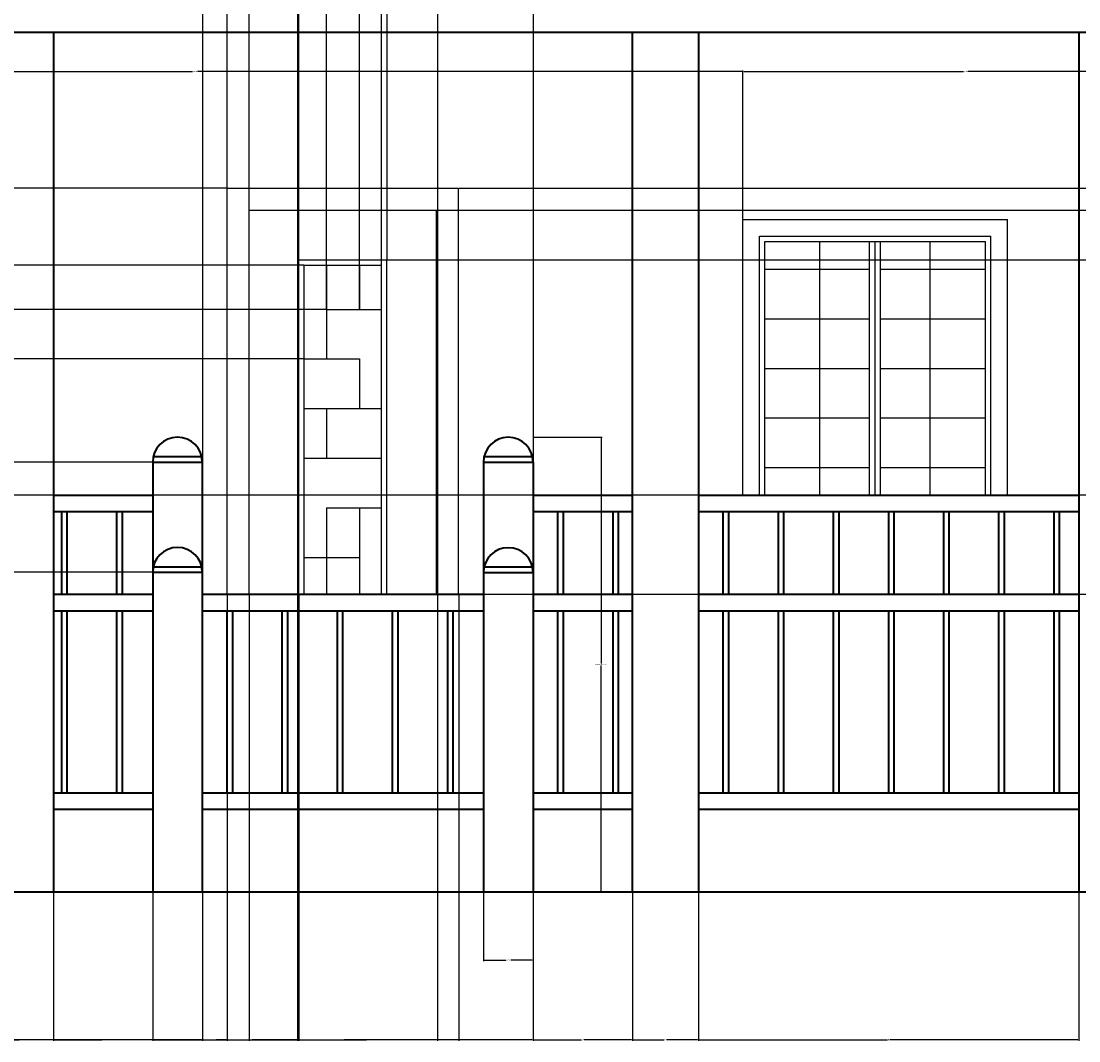
# Model space of a CAD drawing. Units: inches. Extents: x 2154 to 2740, y 571 to 1084.
# Tile 6 of 13: x 2384 to 2576, y 571 to 756. Entities that reach past the tile are written whole.
import ezdxf

# ---------------------------------------------------------------- set-up
doc = ezdxf.new("R2010")
doc.units = ezdxf.units.IN
for name, color, linetype, lineweight in [('A-ANNO-DIMS', 2, 'Continuous', 18), ('A-DOOR', 3, 'Continuous', 25), ('A-ELEV', 7, 'Continuous', 35), ('A-GLAZ', 4, 'Continuous', 25)]:
    doc.layers.add(name, color=color, linetype=linetype, lineweight=lineweight)
doc.styles.get("Standard").update_dxf_attribs({"font": 'arial.ttf'})
doc.dimstyles.get("Standard").update_dxf_attribs({"dimtxt": 0.18, "dimasz": 0.18, "dimexe": 0.18, "dimexo": 0.0625, "dimgap": 0.09, "dimtad": 0, "dimtih": 1, "dimtoh": 1, "dimdec": 4, "dimzin": 0, "dimdsep": 46, "dimtxsty": 'Standard', "dimcen": 0.09, "dimadec": 0, "dimazin": 0, "dimtfac": 1, "dimtdec": 4, "dimtofl": 0, "dimtmove": 0, "dimatfit": 3, "dimfxl": 1, "dimtolj": 1, "dimtzin": 0, "dimarcsym": 0})

# ---------------------------------------------------------------- blocks, each defined once
blk = doc.blocks.new('WIN-ELEV-1200')
for p, q in [((0, 50), (48, 50)), ((0, 0), (0, 50)), ((48, 0), (48, 50)), ((3, 0), (3, 47)), ((3, 47), (45, 47)), ((45, 0), (45, 47)), ((4, 46), (44, 46)), ((4, 0), (4, 46)), ((14, 0), (14, 46)), ((23, 0), (23, 46)), ((24, 0), (24, 46)), ((25, 0), (25, 46)), ((34, 0), (34, 46)), ((44, 0), (44, 46)), ((4, 41), (23, 41)), ((25, 41), (44, 41)), ((4, 32), (23, 32)), ((25, 32), (44, 32)), ((4, 23), (23, 23)), ((25, 23), (44, 23)), ((4, 14), (23, 14)), ((25, 14), (44, 14)), ((4, 5), (23, 5)), ((25, 5), (44, 5))]:
    blk.add_line(p, q)
blk = doc.blocks.new('GATE-POST')
for p, q in [((0, 78), (0, 0)), ((0, 78), (9, 78)), ((9, 78), (9, 0))]:
    blk.add_line(p, q)
blk.add_arc((4.5, 78), 4.5, 0, 180)
blk = doc.blocks.new('*D5')
at = {"layer": 'A-ANNO-DIMS', "color": 0, "lineweight": -2, "transparency": 16777216}
for p, q in [((2477.27, 680.03), (2489.76, 680.03)), ((2489.58, 679.85), (2489.58, 638.97)), ((2489.58, 597.71), (2489.58, 638.6)), ((2477.27, 597.53), (2489.76, 597.53))]:
    blk.add_line(p, q, dxfattribs=at)
at = {"layer": 'A-ANNO-DIMS', "color": 0, "transparency": 16777216}
for points in [[(2489.55, 679.85), (2489.61, 679.85), (2489.58, 680.03)], [(2489.55, 597.71), (2489.61, 597.71), (2489.58, 597.53)]]:
    blk.add_solid(points, dxfattribs=at)
at = {"layer": 'Defpoints', "color": 0, "transparency": 16777216}
for p in [(2477.21, 680.03), (2489.58, 680.03), (2477.21, 597.53)]:
    blk.add_point(p, dxfattribs=at)
at = {"layer": 'A-ANNO-DIMS', "color": 0, "transparency": 16777216, "insert": (2489.58, 638.78), "char_height": 0.18, "attachment_point": 5}
blk.add_mtext('\\A1;GATE POST 83 TYP.', dxfattribs=at)
blk = doc.blocks.new('*D6')
at = {"layer": 'A-ANNO-DIMS', "color": 0, "lineweight": -2, "transparency": 16777216}
for p, q in [((2468.21, 597.47), (2468.21, 584.98)), ((2477.21, 597.47), (2477.21, 584.98)), ((2468.39, 585.16), (2472.25, 585.16)), ((2477.03, 585.16), (2473.16, 585.16))]:
    blk.add_line(p, q, dxfattribs=at)
at = {"layer": 'A-ANNO-DIMS', "color": 0, "transparency": 16777216}
for points in [[(2468.39, 585.19), (2468.39, 585.13), (2468.21, 585.16)], [(2477.03, 585.19), (2477.03, 585.13), (2477.21, 585.16)]]:
    blk.add_solid(points, dxfattribs=at)
at = {"layer": 'Defpoints', "color": 0, "transparency": 16777216}
for p in [(2468.21, 597.53), (2477.21, 597.53), (2477.21, 585.16)]:
    blk.add_point(p, dxfattribs=at)
at = {"layer": 'A-ANNO-DIMS', "color": 0, "transparency": 16777216, "insert": (2472.71, 585.16), "char_height": 0.18, "attachment_point": 5}
blk.add_mtext('\\A1;9 TYP.', dxfattribs=at)
blk = doc.blocks.new('*D9')
at = {"layer": 'A-ANNO-DIMS', "color": 0, "lineweight": -2, "transparency": 16777216}
for p, q in [((2417.21, 970.47), (2417.21, 570.5)), ((2477.21, 970.47), (2477.21, 570.5)), ((2417.39, 570.68), (2446.99, 570.68)), ((2477.03, 570.68), (2447.43, 570.68))]:
    blk.add_line(p, q, dxfattribs=at)
at = {"layer": 'A-ANNO-DIMS', "color": 0, "transparency": 16777216}
for points in [[(2417.39, 570.71), (2417.39, 570.65), (2417.21, 570.68)], [(2477.03, 570.71), (2477.03, 570.65), (2477.21, 570.68)]]:
    blk.add_solid(points, dxfattribs=at)
at = {"layer": 'Defpoints', "color": 0, "transparency": 16777216}
for p in [(2417.21, 970.53), (2477.21, 970.53), (2477.21, 570.68)]:
    blk.add_point(p, dxfattribs=at)
at = {"layer": 'A-ANNO-DIMS', "color": 0, "transparency": 16777216, "insert": (2447.21, 570.68), "char_height": 0.18, "attachment_point": 5}
blk.add_mtext('\\A1;60', dxfattribs=at)
blk = doc.blocks.new('*D10')
at = {"layer": 'A-ANNO-DIMS', "color": 0, "lineweight": -2, "transparency": 16777216}
for p, q in [((2447.14, 1057.01), (2154.18, 1057.01)), ((2154.36, 1056.83), (2154.36, 827.45)), ((2154.36, 597.71), (2154.36, 827.09)), ((2181.14, 597.53), (2154.18, 597.53))]:
    blk.add_line(p, q, dxfattribs=at)
at = {"layer": 'A-ANNO-DIMS', "color": 0, "transparency": 16777216}
for points in [[(2154.33, 1056.83), (2154.39, 1056.83), (2154.36, 1057.01)], [(2154.33, 597.71), (2154.39, 597.71), (2154.36, 597.53)]]:
    blk.add_solid(points, dxfattribs=at)
at = {"layer": 'Defpoints', "color": 0, "transparency": 16777216}
for p in [(2154.36, 1057.01), (2447.21, 1057.01), (2181.21, 597.53)]:
    blk.add_point(p, dxfattribs=at)
at = {"layer": 'A-ANNO-DIMS', "color": 0, "transparency": 16777216, "insert": (2154.36, 827.27), "char_height": 0.18, "attachment_point": 5}
blk.add_mtext('\\A1;459.5', dxfattribs=at)
blk = doc.blocks.new('*D20')
at = {"layer": 'A-ANNO-DIMS', "color": 0, "lineweight": -2, "transparency": 16777216}
for p, q in [((2378.21, 597.47), (2378.21, 570.5)), ((2390.21, 597.47), (2390.21, 570.5)), ((2378.39, 570.68), (2384, 570.68)), ((2390.03, 570.68), (2384.42, 570.68))]:
    blk.add_line(p, q, dxfattribs=at)
at = {"layer": 'A-ANNO-DIMS', "color": 0, "transparency": 16777216}
for points in [[(2378.39, 570.71), (2378.39, 570.65), (2378.21, 570.68)], [(2390.03, 570.71), (2390.03, 570.65), (2390.21, 570.68)]]:
    blk.add_solid(points, dxfattribs=at)
at = {"layer": 'Defpoints', "color": 0, "transparency": 16777216}
for p in [(2378.21, 597.53), (2390.21, 597.53), (2390.21, 570.68)]:
    blk.add_point(p, dxfattribs=at)
at = {"layer": 'A-ANNO-DIMS', "color": 0, "transparency": 16777216, "insert": (2384.21, 570.68), "char_height": 0.18, "attachment_point": 5}
blk.add_mtext('\\A1;12', dxfattribs=at)
blk = doc.blocks.new('*D21')
at = {"layer": 'A-ANNO-DIMS', "color": 0, "lineweight": -2, "transparency": 16777216}
for p, q in [((2390.21, 597.47), (2390.21, 570.5)), ((2408.21, 597.47), (2408.21, 570.5)), ((2390.39, 570.68), (2399, 570.68)), ((2408.03, 570.68), (2399.42, 570.68))]:
    blk.add_line(p, q, dxfattribs=at)
at = {"layer": 'A-ANNO-DIMS', "color": 0, "transparency": 16777216}
for points in [[(2390.39, 570.71), (2390.39, 570.65), (2390.21, 570.68)], [(2408.03, 570.71), (2408.03, 570.65), (2408.21, 570.68)]]:
    blk.add_solid(points, dxfattribs=at)
at = {"layer": 'Defpoints', "color": 0, "transparency": 16777216}
for p in [(2390.21, 597.53), (2408.21, 597.53), (2408.21, 570.68)]:
    blk.add_point(p, dxfattribs=at)
at = {"layer": 'A-ANNO-DIMS', "color": 0, "transparency": 16777216, "insert": (2399.21, 570.68), "char_height": 0.18, "attachment_point": 5}
blk.add_mtext('\\A1;18', dxfattribs=at)
blk = doc.blocks.new('*D22')
at = {"layer": 'A-ANNO-DIMS', "color": 0, "lineweight": -2, "transparency": 16777216}
for p, q in [((2408.21, 597.47), (2408.21, 570.5)), ((2477.21, 597.47), (2477.21, 570.5)), ((2408.39, 570.68), (2442.49, 570.68)), ((2477.03, 570.68), (2442.93, 570.68))]:
    blk.add_line(p, q, dxfattribs=at)
at = {"layer": 'A-ANNO-DIMS', "color": 0, "transparency": 16777216}
for points in [[(2408.39, 570.71), (2408.39, 570.65), (2408.21, 570.68)], [(2477.03, 570.71), (2477.03, 570.65), (2477.21, 570.68)]]:
    blk.add_solid(points, dxfattribs=at)
at = {"layer": 'Defpoints', "color": 0, "transparency": 16777216}
for p in [(2408.21, 597.53), (2477.21, 597.53), (2477.21, 570.68)]:
    blk.add_point(p, dxfattribs=at)
at = {"layer": 'A-ANNO-DIMS', "color": 0, "transparency": 16777216, "insert": (2442.71, 570.68), "char_height": 0.18, "attachment_point": 5}
blk.add_mtext('\\A1;69', dxfattribs=at)
blk = doc.blocks.new('*D23')
at = {"layer": 'A-ANNO-DIMS', "color": 0, "lineweight": -2, "transparency": 16777216}
for p, q in [((2477.21, 597.47), (2477.21, 570.5)), ((2495.21, 597.47), (2495.21, 570.5)), ((2477.39, 570.68), (2486, 570.68)), ((2495.03, 570.68), (2486.42, 570.68))]:
    blk.add_line(p, q, dxfattribs=at)
at = {"layer": 'A-ANNO-DIMS', "color": 0, "transparency": 16777216}
for points in [[(2477.39, 570.71), (2477.39, 570.65), (2477.21, 570.68)], [(2495.03, 570.71), (2495.03, 570.65), (2495.21, 570.68)]]:
    blk.add_solid(points, dxfattribs=at)
at = {"layer": 'Defpoints', "color": 0, "transparency": 16777216}
for p in [(2477.21, 597.53), (2495.21, 597.53), (2495.21, 570.68)]:
    blk.add_point(p, dxfattribs=at)
at = {"layer": 'A-ANNO-DIMS', "color": 0, "transparency": 16777216, "insert": (2486.21, 570.68), "char_height": 0.18, "attachment_point": 5}
blk.add_mtext('\\A1;18', dxfattribs=at)
blk = doc.blocks.new('*D24')
at = {"layer": 'A-ANNO-DIMS', "color": 0, "lineweight": -2, "transparency": 16777216}
for p, q in [((2495.21, 597.47), (2495.21, 570.5)), ((2507.21, 597.47), (2507.21, 570.5)), ((2495.39, 570.68), (2501, 570.68)), ((2507.03, 570.68), (2501.42, 570.68))]:
    blk.add_line(p, q, dxfattribs=at)
at = {"layer": 'A-ANNO-DIMS', "color": 0, "transparency": 16777216}
for points in [[(2495.39, 570.71), (2495.39, 570.65), (2495.21, 570.68)], [(2507.03, 570.71), (2507.03, 570.65), (2507.21, 570.68)]]:
    blk.add_solid(points, dxfattribs=at)
at = {"layer": 'Defpoints', "color": 0, "transparency": 16777216}
for p in [(2495.21, 597.53), (2507.21, 597.53), (2507.21, 570.68)]:
    blk.add_point(p, dxfattribs=at)
at = {"layer": 'A-ANNO-DIMS', "color": 0, "transparency": 16777216, "insert": (2501.21, 570.68), "char_height": 0.18, "attachment_point": 5}
blk.add_mtext('\\A1;12', dxfattribs=at)
blk = doc.blocks.new('*D25')
at = {"layer": 'A-ANNO-DIMS', "color": 0, "lineweight": -2, "transparency": 16777216}
for p, q in [((2507.21, 597.47), (2507.21, 570.5)), ((2576.21, 597.47), (2576.21, 570.5)), ((2507.39, 570.68), (2541.49, 570.68)), ((2576.03, 570.68), (2541.93, 570.68))]:
    blk.add_line(p, q, dxfattribs=at)
at = {"layer": 'A-ANNO-DIMS', "color": 0, "transparency": 16777216}
for points in [[(2507.39, 570.71), (2507.39, 570.65), (2507.21, 570.68)], [(2576.03, 570.71), (2576.03, 570.65), (2576.21, 570.68)]]:
    blk.add_solid(points, dxfattribs=at)
at = {"layer": 'Defpoints', "color": 0, "transparency": 16777216}
for p in [(2507.21, 597.53), (2576.21, 597.53), (2576.21, 570.68)]:
    blk.add_point(p, dxfattribs=at)
at = {"layer": 'A-ANNO-DIMS', "color": 0, "transparency": 16777216, "insert": (2541.71, 570.68), "char_height": 0.18, "attachment_point": 5}
blk.add_mtext('\\A1;69', dxfattribs=at)
blk = doc.blocks.new('*D29')
at = {"layer": 'A-ANNO-DIMS', "color": 0, "lineweight": -2, "transparency": 16777216}
for p, q in [((2657.14, 669.53), (2154.18, 669.53)), ((2154.36, 669.35), (2154.36, 633.71)), ((2154.36, 597.71), (2154.36, 633.35)), ((2657.14, 597.53), (2154.18, 597.53))]:
    blk.add_line(p, q, dxfattribs=at)
at = {"layer": 'A-ANNO-DIMS', "color": 0, "transparency": 16777216}
for points in [[(2154.33, 669.35), (2154.39, 669.35), (2154.36, 669.53)], [(2154.33, 597.71), (2154.39, 597.71), (2154.36, 597.53)]]:
    blk.add_solid(points, dxfattribs=at)
at = {"layer": 'Defpoints', "color": 0, "transparency": 16777216}
for p in [(2154.36, 669.53), (2657.21, 669.53), (2657.21, 597.53)]:
    blk.add_point(p, dxfattribs=at)
at = {"layer": 'A-ANNO-DIMS', "color": 0, "transparency": 16777216, "insert": (2154.36, 633.53), "char_height": 0.18, "attachment_point": 5}
blk.add_mtext('\\A1;72', dxfattribs=at)
blk = doc.blocks.new('*D31')
at = {"layer": 'A-ANNO-DIMS', "color": 0, "lineweight": -2, "transparency": 16777216}
for p, q in [((2421.64, 725.23), (2154.18, 725.23)), ((2154.36, 725.05), (2154.36, 661.56)), ((2154.36, 597.71), (2154.36, 661.2)), ((2417.14, 597.53), (2154.18, 597.53))]:
    blk.add_line(p, q, dxfattribs=at)
at = {"layer": 'A-ANNO-DIMS', "color": 0, "transparency": 16777216}
for points in [[(2154.33, 725.05), (2154.39, 725.05), (2154.36, 725.23)], [(2154.33, 597.71), (2154.39, 597.71), (2154.36, 597.53)]]:
    blk.add_solid(points, dxfattribs=at)
at = {"layer": 'Defpoints', "color": 0, "transparency": 16777216}
for p in [(2154.36, 725.23), (2421.71, 725.23), (2417.21, 597.53)]:
    blk.add_point(p, dxfattribs=at)
at = {"layer": 'A-ANNO-DIMS', "color": 0, "transparency": 16777216, "insert": (2154.36, 661.38), "char_height": 0.18, "attachment_point": 5}
blk.add_mtext('\\A1;127.7', dxfattribs=at)
blk = doc.blocks.new('*D39')
at = {"layer": 'A-ANNO-DIMS', "color": 0, "lineweight": -2, "transparency": 16777216}
for p, q in [((2183.21, 979.47), (2183.21, 570.5)), ((2417.21, 970.47), (2417.21, 570.5)), ((2183.39, 570.68), (2299.92, 570.68)), ((2417.03, 570.68), (2300.5, 570.68))]:
    blk.add_line(p, q, dxfattribs=at)
at = {"layer": 'A-ANNO-DIMS', "color": 0, "transparency": 16777216}
for points in [[(2183.39, 570.71), (2183.39, 570.65), (2183.21, 570.68)], [(2417.03, 570.71), (2417.03, 570.65), (2417.21, 570.68)]]:
    blk.add_solid(points, dxfattribs=at)
at = {"layer": 'Defpoints', "color": 0, "transparency": 16777216}
for p in [(2183.21, 979.53), (2417.21, 970.53), (2417.21, 570.68)]:
    blk.add_point(p, dxfattribs=at)
at = {"layer": 'A-ANNO-DIMS', "color": 0, "transparency": 16777216, "insert": (2300.21, 570.68), "char_height": 0.18, "attachment_point": 5}
blk.add_mtext('\\A1;234', dxfattribs=at)
blk = doc.blocks.new('*D44')
at = {"layer": 'A-ANNO-DIMS', "color": 0, "lineweight": -2, "transparency": 16777216}
for p, q in [((2316.5, 719.59), (2316.5, 746.56)), ((2316.68, 746.38), (2415.42, 746.38)), ((2515.07, 746.38), (2416.33, 746.38)), ((2515.25, 719.59), (2515.25, 746.56))]:
    blk.add_line(p, q, dxfattribs=at)
at = {"layer": 'A-ANNO-DIMS', "color": 0, "transparency": 16777216}
for points in [[(2316.68, 746.41), (2316.68, 746.35), (2316.5, 746.38)], [(2515.07, 746.41), (2515.07, 746.35), (2515.25, 746.38)]]:
    blk.add_solid(points, dxfattribs=at)
at = {"layer": 'Defpoints', "color": 0, "transparency": 16777216}
for p in [(2515.25, 746.38), (2316.5, 719.53), (2515.25, 719.53)]:
    blk.add_point(p, dxfattribs=at)
at = {"layer": 'A-ANNO-DIMS', "color": 0, "transparency": 16777216, "insert": (2415.87, 746.38), "char_height": 0.18, "attachment_point": 5}
blk.add_mtext('\\A1;198.75', dxfattribs=at)
blk = doc.blocks.new('*D45')
at = {"layer": 'A-ANNO-DIMS', "color": 0, "lineweight": -2, "transparency": 16777216}
for p, q in [((2515.25, 719.59), (2515.25, 746.56)), ((2515.43, 746.38), (2555.29, 746.38)), ((2595.93, 746.38), (2556.07, 746.38)), ((2596.11, 719.59), (2596.11, 746.56))]:
    blk.add_line(p, q, dxfattribs=at)
at = {"layer": 'A-ANNO-DIMS', "color": 0, "transparency": 16777216}
for points in [[(2515.43, 746.41), (2515.43, 746.35), (2515.25, 746.38)], [(2595.93, 746.41), (2595.93, 746.35), (2596.11, 746.38)]]:
    blk.add_solid(points, dxfattribs=at)
at = {"layer": 'Defpoints', "color": 0, "transparency": 16777216}
for p in [(2596.11, 746.38), (2515.25, 719.53), (2596.11, 719.53)]:
    blk.add_point(p, dxfattribs=at)
at = {"layer": 'A-ANNO-DIMS', "color": 0, "transparency": 16777216, "insert": (2555.68, 746.38), "char_height": 0.18, "attachment_point": 5}
blk.add_mtext('\\A1;80.86', dxfattribs=at)
blk = doc.blocks.new('*D75')
at = {"layer": 'A-ANNO-DIMS', "color": 0, "lineweight": -2, "transparency": 16777216}
for p, q in [((2434.46, 990.57), (2434.46, 570.5)), ((2417.21, 981.47), (2417.21, 570.5)), ((2417.39, 570.68), (2425.45, 570.68)), ((2434.28, 570.68), (2426.22, 570.68))]:
    blk.add_line(p, q, dxfattribs=at)
at = {"layer": 'A-ANNO-DIMS', "color": 0, "transparency": 16777216}
for points in [[(2417.39, 570.71), (2417.39, 570.65), (2417.21, 570.68)], [(2434.28, 570.71), (2434.28, 570.65), (2434.46, 570.68)]]:
    blk.add_solid(points, dxfattribs=at)
at = {"layer": 'Defpoints', "color": 0, "transparency": 16777216}
for p in [(2434.46, 990.64), (2417.21, 981.53), (2434.46, 570.68)]:
    blk.add_point(p, dxfattribs=at)
at = {"layer": 'A-ANNO-DIMS', "color": 0, "transparency": 16777216, "insert": (2425.83, 570.68), "char_height": 0.18, "attachment_point": 5}
blk.add_mtext('\\A1;17.25', dxfattribs=at)
blk = doc.blocks.new('*D76')
at = {"layer": 'A-ANNO-DIMS', "color": 0, "lineweight": -2, "transparency": 16777216}
for p, q in [((2434.46, 990.57), (2434.46, 570.5)), ((2459.89, 990.57), (2459.89, 570.5)), ((2434.64, 570.68), (2446.71, 570.68)), ((2459.71, 570.68), (2447.64, 570.68))]:
    blk.add_line(p, q, dxfattribs=at)
at = {"layer": 'A-ANNO-DIMS', "color": 0, "transparency": 16777216}
for points in [[(2434.64, 570.71), (2434.64, 570.65), (2434.46, 570.68)], [(2459.71, 570.71), (2459.71, 570.65), (2459.89, 570.68)]]:
    blk.add_solid(points, dxfattribs=at)
at = {"layer": 'Defpoints', "color": 0, "transparency": 16777216}
for p in [(2434.46, 990.64), (2459.89, 990.64), (2459.89, 570.68)]:
    blk.add_point(p, dxfattribs=at)
at = {"layer": 'A-ANNO-DIMS', "color": 0, "transparency": 16777216, "insert": (2447.17, 570.68), "char_height": 0.18, "attachment_point": 5}
blk.add_mtext('\\A1;25.433', dxfattribs=at)
blk = doc.blocks.new('*D86')
at = {"layer": 'A-ANNO-DIMS', "color": 0, "lineweight": -2, "transparency": 16777216}
for p, q in [((2421.71, 651.47), (2421.71, 570.5)), ((2463.71, 651.47), (2463.71, 570.5)), ((2421.89, 570.68), (2442.49, 570.68)), ((2463.53, 570.68), (2442.93, 570.68))]:
    blk.add_line(p, q, dxfattribs=at)
at = {"layer": 'A-ANNO-DIMS', "color": 0, "transparency": 16777216}
for points in [[(2421.89, 570.71), (2421.89, 570.65), (2421.71, 570.68)], [(2463.53, 570.71), (2463.53, 570.65), (2463.71, 570.68)]]:
    blk.add_solid(points, dxfattribs=at)
at = {"layer": 'Defpoints', "color": 0, "transparency": 16777216}
for p in [(2421.71, 651.53), (2463.71, 651.53), (2463.71, 570.68)]:
    blk.add_point(p, dxfattribs=at)
at = {"layer": 'A-ANNO-DIMS', "color": 0, "transparency": 16777216, "insert": (2442.71, 570.68), "char_height": 0.18, "attachment_point": 5}
blk.add_mtext('\\A1;42', dxfattribs=at)
blk = doc.blocks.new('*D87')
at = {"layer": 'A-ANNO-DIMS', "color": 0, "lineweight": -2, "transparency": 16777216}
for p, q in [((2421.71, 725.29), (2421.71, 1084.04)), ((2425.71, 721.29), (2425.71, 1084.04)), ((2421.89, 1083.86), (2423.55, 1083.86)), ((2425.53, 1083.86), (2423.86, 1083.86))]:
    blk.add_line(p, q, dxfattribs=at)
at = {"layer": 'A-ANNO-DIMS', "color": 0, "transparency": 16777216}
for points in [[(2421.89, 1083.89), (2421.89, 1083.83), (2421.71, 1083.86)], [(2425.53, 1083.89), (2425.53, 1083.83), (2425.71, 1083.86)]]:
    blk.add_solid(points, dxfattribs=at)
at = {"layer": 'Defpoints', "color": 0, "transparency": 16777216}
for p in [(2425.71, 1083.86), (2421.71, 725.23), (2425.71, 721.23)]:
    blk.add_point(p, dxfattribs=at)
at = {"layer": 'A-ANNO-DIMS', "color": 0, "transparency": 16777216, "insert": (2423.71, 1083.86), "char_height": 0.18, "attachment_point": 5}
blk.add_mtext('\\A1;4', dxfattribs=at)
blk = doc.blocks.new('*D88')
at = {"layer": 'A-ANNO-DIMS', "color": 0, "lineweight": -2, "transparency": 16777216}
for p, q in [((2463.769199, 725.228066), (2740.236699, 725.228066)), ((2740.056699, 725.048066), (2740.056699, 723.408066)), ((2740.056699, 721.408066), (2740.056699, 723.048066)), ((2459.769199, 721.228066), (2740.236699, 721.228066))]:
    blk.add_line(p, q, dxfattribs=at)
at = {"layer": 'A-ANNO-DIMS', "color": 0, "transparency": 16777216}
for points in [[(2740.026699, 725.048066), (2740.086699, 725.048066), (2740.056699, 725.228066)], [(2740.026699, 721.408066), (2740.086699, 721.408066), (2740.056699, 721.228066)]]:
    blk.add_solid(points, dxfattribs=at)
at = {"layer": 'Defpoints', "color": 0, "transparency": 16777216}
for p in [(2463.706699, 725.228066), (2740.056699, 725.228066), (2459.706699, 721.228066)]:
    blk.add_point(p, dxfattribs=at)
at = {"layer": 'A-ANNO-DIMS', "color": 0, "transparency": 16777216, "insert": (2740.056699, 723.228066), "char_height": 0.18, "attachment_point": 5}
blk.add_mtext('\\A1;4', dxfattribs=at)
blk = doc.blocks.new('*D89')
at = {"layer": 'A-ANNO-DIMS', "color": 0, "lineweight": -2, "transparency": 16777216}
for p, q in [((2425.71, 651.47), (2425.71, 570.5)), ((2434.71, 651.47), (2434.71, 570.5)), ((2425.89, 570.68), (2430.06, 570.68)), ((2434.53, 570.68), (2430.36, 570.68))]:
    blk.add_line(p, q, dxfattribs=at)
at = {"layer": 'A-ANNO-DIMS', "color": 0, "transparency": 16777216}
for points in [[(2425.89, 570.71), (2425.89, 570.65), (2425.71, 570.68)], [(2434.53, 570.71), (2434.53, 570.65), (2434.71, 570.68)]]:
    blk.add_solid(points, dxfattribs=at)
at = {"layer": 'Defpoints', "color": 0, "transparency": 16777216}
for p in [(2425.71, 651.53), (2434.71, 651.53), (2434.71, 570.68)]:
    blk.add_point(p, dxfattribs=at)
at = {"layer": 'A-ANNO-DIMS', "color": 0, "transparency": 16777216, "insert": (2430.21, 570.68), "char_height": 0.18, "attachment_point": 5}
blk.add_mtext('\\A1;9', dxfattribs=at)
blk = doc.blocks.new('*D90')
at = {"layer": 'A-ANNO-DIMS', "color": 0, "lineweight": -2, "transparency": 16777216}
for p, q in [((2434.71, 712.29), (2434.71, 1084.04)), ((2450.71, 712.29), (2450.71, 1084.04)), ((2434.89, 1083.86), (2442.5, 1083.86)), ((2450.53, 1083.86), (2442.92, 1083.86))]:
    blk.add_line(p, q, dxfattribs=at)
at = {"layer": 'A-ANNO-DIMS', "color": 0, "transparency": 16777216}
for points in [[(2434.89, 1083.89), (2434.89, 1083.83), (2434.71, 1083.86)], [(2450.53, 1083.89), (2450.53, 1083.83), (2450.71, 1083.86)]]:
    blk.add_solid(points, dxfattribs=at)
at = {"layer": 'Defpoints', "color": 0, "transparency": 16777216}
for p in [(2450.71, 1083.86), (2434.71, 712.23), (2450.71, 712.23)]:
    blk.add_point(p, dxfattribs=at)
at = {"layer": 'A-ANNO-DIMS', "color": 0, "transparency": 16777216, "insert": (2442.71, 1083.86), "char_height": 0.18, "attachment_point": 5}
blk.add_mtext('\\A1;16', dxfattribs=at)
blk = doc.blocks.new('*D91')
at = {"layer": 'A-ANNO-DIMS', "color": 0, "lineweight": -2, "transparency": 16777216}
for p, q in [((2450.77, 712.23), (2740.24, 712.23)), ((2740.06, 712.05), (2740.06, 682.06)), ((2740.06, 651.71), (2740.06, 681.7)), ((2450.77, 651.53), (2740.24, 651.53))]:
    blk.add_line(p, q, dxfattribs=at)
at = {"layer": 'A-ANNO-DIMS', "color": 0, "transparency": 16777216}
for points in [[(2740.03, 712.05), (2740.09, 712.05), (2740.06, 712.23)], [(2740.03, 651.71), (2740.09, 651.71), (2740.06, 651.53)]]:
    blk.add_solid(points, dxfattribs=at)
at = {"layer": 'Defpoints', "color": 0, "transparency": 16777216}
for p in [(2450.71, 712.23), (2740.06, 712.23), (2450.71, 651.53)]:
    blk.add_point(p, dxfattribs=at)
at = {"layer": 'A-ANNO-DIMS', "color": 0, "transparency": 16777216, "insert": (2740.06, 681.88), "char_height": 0.18, "attachment_point": 5}
blk.add_mtext('\\A1;60.7', dxfattribs=at)
blk = doc.blocks.new('*D92')
at = {"layer": 'A-ANNO-DIMS', "color": 0, "lineweight": -2, "transparency": 16777216}
for p, q in [((2463.77, 725.23), (2740.24, 725.23)), ((2740.06, 725.05), (2740.06, 688.56)), ((2740.06, 651.71), (2740.06, 688.2)), ((2463.77, 651.53), (2740.24, 651.53))]:
    blk.add_line(p, q, dxfattribs=at)
at = {"layer": 'A-ANNO-DIMS', "color": 0, "transparency": 16777216}
for points in [[(2740.03, 725.05), (2740.09, 725.05), (2740.06, 725.23)], [(2740.03, 651.71), (2740.09, 651.71), (2740.06, 651.53)]]:
    blk.add_solid(points, dxfattribs=at)
at = {"layer": 'Defpoints', "color": 0, "transparency": 16777216}
for p in [(2463.71, 725.23), (2740.06, 725.23), (2463.71, 651.53)]:
    blk.add_point(p, dxfattribs=at)
at = {"layer": 'A-ANNO-DIMS', "color": 0, "transparency": 16777216, "insert": (2740.06, 688.38), "char_height": 0.18, "attachment_point": 5}
blk.add_mtext('\\A1;73.7', dxfattribs=at)
blk = doc.blocks.new('*D93')
at = {"layer": 'A-ANNO-DIMS', "color": 0, "lineweight": -2, "transparency": 16777216}
for p, q in [((2439.71, 703.29), (2439.71, 1084.04)), ((2445.71, 703.29), (2445.71, 1084.04)), ((2439.89, 1083.86), (2442.56, 1083.86)), ((2445.53, 1083.86), (2442.86, 1083.86))]:
    blk.add_line(p, q, dxfattribs=at)
at = {"layer": 'A-ANNO-DIMS', "color": 0, "transparency": 16777216}
for points in [[(2439.89, 1083.89), (2439.89, 1083.83), (2439.71, 1083.86)], [(2445.53, 1083.89), (2445.53, 1083.83), (2445.71, 1083.86)]]:
    blk.add_solid(points, dxfattribs=at)
at = {"layer": 'Defpoints', "color": 0, "transparency": 16777216}
for p in [(2445.71, 1083.86), (2439.71, 703.23), (2445.71, 703.23)]:
    blk.add_point(p, dxfattribs=at)
at = {"layer": 'A-ANNO-DIMS', "color": 0, "transparency": 16777216, "insert": (2442.71, 1083.86), "char_height": 0.18, "attachment_point": 5}
blk.add_mtext('\\A1;6', dxfattribs=at)
blk = doc.blocks.new('*D94')
at = {"layer": 'A-ANNO-DIMS', "color": 0, "lineweight": -2, "transparency": 16777216}
for p, q in [((2445.71, 703.29), (2445.71, 1084.04)), ((2449.71, 703.29), (2449.71, 1084.04)), ((2445.89, 1083.86), (2447.55, 1083.86)), ((2449.53, 1083.86), (2447.86, 1083.86))]:
    blk.add_line(p, q, dxfattribs=at)
at = {"layer": 'A-ANNO-DIMS', "color": 0, "transparency": 16777216}
for points in [[(2445.89, 1083.89), (2445.89, 1083.83), (2445.71, 1083.86)], [(2449.53, 1083.89), (2449.53, 1083.83), (2449.71, 1083.86)]]:
    blk.add_solid(points, dxfattribs=at)
at = {"layer": 'Defpoints', "color": 0, "transparency": 16777216}
for p in [(2449.71, 1083.86), (2445.71, 703.23), (2449.71, 703.23)]:
    blk.add_point(p, dxfattribs=at)
at = {"layer": 'A-ANNO-DIMS', "color": 0, "transparency": 16777216, "insert": (2447.71, 1083.86), "char_height": 0.18, "attachment_point": 5}
blk.add_mtext('\\A1;4', dxfattribs=at)
blk = doc.blocks.new('*D95')
at = {"layer": 'A-ANNO-DIMS', "color": 0, "lineweight": -2, "transparency": 16777216}
for p, q in [((2435.64, 711.23), (2154.18, 711.23)), ((2154.36, 711.05), (2154.36, 707.41)), ((2154.36, 703.41), (2154.36, 707.05)), ((2439.64, 703.23), (2154.18, 703.23))]:
    blk.add_line(p, q, dxfattribs=at)
at = {"layer": 'A-ANNO-DIMS', "color": 0, "transparency": 16777216}
for points in [[(2154.33, 711.05), (2154.39, 711.05), (2154.36, 711.23)], [(2154.33, 703.41), (2154.39, 703.41), (2154.36, 703.23)]]:
    blk.add_solid(points, dxfattribs=at)
at = {"layer": 'Defpoints', "color": 0, "transparency": 16777216}
for p in [(2435.71, 711.23), (2154.36, 703.23), (2439.71, 703.23)]:
    blk.add_point(p, dxfattribs=at)
at = {"layer": 'A-ANNO-DIMS', "color": 0, "transparency": 16777216, "insert": (2154.36, 707.23), "char_height": 0.18, "attachment_point": 5}
blk.add_mtext('\\A1;8', dxfattribs=at)
blk = doc.blocks.new('*D96')
at = {"layer": 'A-ANNO-DIMS', "color": 0, "lineweight": -2, "transparency": 16777216}
for p, q in [((2439.64, 703.23), (2154.18, 703.23)), ((2154.36, 703.05), (2154.36, 698.91)), ((2154.36, 694.41), (2154.36, 698.55)), ((2435.64, 694.23), (2154.18, 694.23))]:
    blk.add_line(p, q, dxfattribs=at)
at = {"layer": 'A-ANNO-DIMS', "color": 0, "transparency": 16777216}
for points in [[(2154.33, 703.05), (2154.39, 703.05), (2154.36, 703.23)], [(2154.33, 694.41), (2154.39, 694.41), (2154.36, 694.23)]]:
    blk.add_solid(points, dxfattribs=at)
at = {"layer": 'Defpoints', "color": 0, "transparency": 16777216}
for p in [(2439.71, 703.23), (2154.36, 694.23), (2435.71, 694.23)]:
    blk.add_point(p, dxfattribs=at)
at = {"layer": 'A-ANNO-DIMS', "color": 0, "transparency": 16777216, "insert": (2154.36, 698.73), "char_height": 0.18, "attachment_point": 5}
blk.add_mtext('\\A1;9', dxfattribs=at)
blk = doc.blocks.new('*D97')
at = {"layer": 'A-ANNO-DIMS', "color": 0, "lineweight": -2, "transparency": 16777216}
for p, q in [((2417.21, 675.47), (2417.21, 570.5)), ((2421.71, 651.47), (2421.71, 570.5)), ((2417.39, 570.68), (2419.2, 570.68)), ((2421.53, 570.68), (2419.71, 570.68))]:
    blk.add_line(p, q, dxfattribs=at)
at = {"layer": 'A-ANNO-DIMS', "color": 0, "transparency": 16777216}
for points in [[(2417.39, 570.71), (2417.39, 570.65), (2417.21, 570.68)], [(2421.53, 570.71), (2421.53, 570.65), (2421.71, 570.68)]]:
    blk.add_solid(points, dxfattribs=at)
at = {"layer": 'Defpoints', "color": 0, "transparency": 16777216}
for p in [(2417.21, 675.53), (2421.71, 651.53), (2421.71, 570.68)]:
    blk.add_point(p, dxfattribs=at)
at = {"layer": 'A-ANNO-DIMS', "color": 0, "transparency": 16777216, "insert": (2419.46, 570.68), "char_height": 0.18, "attachment_point": 5}
blk.add_mtext('\\A1;4.5', dxfattribs=at)
blk = doc.blocks.new('*D98')
at = {"layer": 'A-ANNO-DIMS', "color": 0, "lineweight": -2, "transparency": 16777216}
for p, q in [((2408.14, 675.53), (2154.18, 675.53)), ((2154.36, 675.35), (2154.36, 665.71)), ((2154.36, 655.71), (2154.36, 665.35)), ((2408.14, 655.53), (2154.18, 655.53))]:
    blk.add_line(p, q, dxfattribs=at)
at = {"layer": 'A-ANNO-DIMS', "color": 0, "transparency": 16777216}
for points in [[(2154.33, 675.35), (2154.39, 675.35), (2154.36, 675.53)], [(2154.33, 655.71), (2154.39, 655.71), (2154.36, 655.53)]]:
    blk.add_solid(points, dxfattribs=at)
at = {"layer": 'Defpoints', "color": 0, "transparency": 16777216}
for p in [(2154.36, 675.53), (2408.21, 675.53), (2408.21, 655.53)]:
    blk.add_point(p, dxfattribs=at)
at = {"layer": 'A-ANNO-DIMS', "color": 0, "transparency": 16777216, "insert": (2154.36, 665.53), "char_height": 0.18, "attachment_point": 5}
blk.add_mtext('\\A1;20', dxfattribs=at)

msp = doc.modelspace()

# ---------------------------------------------------------------- linework, layer by layer
at = {"layer": 'A-DOOR'}
for p, q in [((2421.7067, 651.5321), (2421.7067, 725.2281)), ((2421.7067, 725.2281), (2463.7067, 725.2281)), ((2463.7067, 651.5321), (2463.7067, 725.2281)), ((2425.7067, 721.2281), (2459.7067, 721.2281)), ((2425.7067, 651.5321), (2425.7067, 721.2281)), ((2459.7067, 651.5321), (2459.7067, 721.2281)), ((2434.7067, 651.5321), (2434.7067, 712.2281)), ((2434.7067, 712.2281), (2450.7067, 712.2281)), ((2450.7067, 651.5321), (2450.7067, 712.2281)), ((2435.7067, 711.2281), (2449.7067, 711.2281)), ((2435.7067, 651.5321), (2435.7067, 711.2281)), ((2439.7067, 711.2281), (2439.7067, 694.2281)), ((2445.7067, 711.2281), (2445.7067, 703.2281)), ((2449.7067, 651.5321), (2449.7067, 711.2281)), ((2439.7067, 703.2281), (2449.7067, 703.2281)), ((2435.7067, 694.2281), (2445.7067, 694.2281)), ((2445.7067, 694.2281), (2445.7067, 685.2281)), ((2435.7067, 685.2281), (2449.7067, 685.2281)), ((2439.7067, 685.2281), (2439.7067, 676.2281)), ((2435.7067, 676.2281), (2449.7067, 676.2281)), ((2439.7067, 667.2281), (2449.7067, 667.2281)), ((2439.7067, 667.2281), (2439.7067, 651.5321)), ((2445.7067, 667.2281), (2445.7067, 651.5321)), ((2435.7067, 658.2281), (2445.7067, 658.2281))]:
    msp.add_line(p, q, dxfattribs=at)
at = {"layer": 'A-ELEV'}
for p, q in [((2181.2067, 753.5321), (2713.2067, 753.5321)), ((2390.2067, 753.5321), (2390.2067, 597.5321)), ((2495.2067, 753.5321), (2495.2067, 597.5321)), ((2507.2067, 753.5321), (2507.2067, 597.5321)), ((2576.2067, 753.5321), (2576.2067, 597.5321)), ((2408.2067, 676.5321), (2417.2067, 676.5321)), ((2468.2067, 676.5321), (2477.2067, 676.5321)), ((2390.2067, 669.5321), (2408.2067, 669.5321)), ((2477.2067, 669.5321), (2495.2067, 669.5321)), ((2507.2067, 669.5321), (2576.2067, 669.5321)), ((2390.2067, 666.5321), (2408.2067, 666.5321)), ((2391.6527, 666.5321), (2391.6527, 651.5321)), ((2392.6527, 666.5321), (2392.6527, 651.5321)), ((2401.6527, 666.5321), (2401.6527, 651.5321)), ((2402.6527, 666.5321), (2402.6527, 651.5321)), ((2477.2067, 666.5321), (2495.2067, 666.5321)), ((2481.6527, 666.5321), (2481.6527, 651.5321)), ((2482.6527, 666.5321), (2482.6527, 651.5321)), ((2491.6527, 666.5321), (2491.6527, 651.5321)), ((2492.6527, 666.5321), (2492.6527, 651.5321)), ((2507.2067, 666.5321), (2576.2067, 666.5321)), ((2511.6527, 666.5321), (2511.6527, 651.5321)), ((2512.6527, 666.5321), (2512.6527, 651.5321)), ((2521.6527, 666.5321), (2521.6527, 651.5321)), ((2522.6527, 666.5321), (2522.6527, 651.5321)), ((2531.6527, 666.5321), (2531.6527, 651.5321)), ((2532.6527, 666.5321), (2532.6527, 651.5321)), ((2541.6527, 666.5321), (2541.6527, 651.5321)), ((2542.6527, 666.5321), (2542.6527, 651.5321)), ((2551.6527, 666.5321), (2551.6527, 651.5321)), ((2552.6527, 666.5321), (2552.6527, 651.5321)), ((2561.6527, 666.5321), (2561.6527, 651.5321)), ((2562.6527, 666.5321), (2562.6527, 651.5321)), ((2571.6527, 666.5321), (2571.6527, 651.5321)), ((2572.6527, 666.5321), (2572.6527, 651.5321)), ((2408.2067, 656.5321), (2417.2067, 656.5321)), ((2468.2067, 656.4869), (2477.2067, 656.4869)), ((2408.2067, 655.5321), (2417.2067, 655.5321)), ((2468.2067, 655.4869), (2477.2067, 655.4869)), ((2390.2067, 651.5321), (2408.2067, 651.5321)), ((2417.2067, 651.5321), (2468.2067, 651.5321)), ((2477.2067, 651.5321), (2495.2067, 651.5321)), ((2507.2067, 651.5321), (2576.2067, 651.5321)), ((2390.2067, 648.5321), (2408.2067, 648.5321)), ((2391.6527, 648.5321), (2391.6527, 615.5321)), ((2392.6527, 648.5321), (2392.6527, 615.5321)), ((2401.6527, 648.5321), (2401.6527, 615.5321)), ((2402.6527, 648.5321), (2402.6527, 615.5321)), ((2417.2067, 648.5321), (2468.2067, 648.5321)), ((2421.6527, 648.5321), (2421.6527, 615.5321)), ((2422.6527, 648.5321), (2422.6527, 615.5321)), ((2431.6527, 648.5321), (2431.6527, 615.5321)), ((2432.6527, 648.5321), (2432.6527, 615.5321)), ((2441.6527, 648.5321), (2441.6527, 615.5321)), ((2442.6527, 648.5321), (2442.6527, 615.5321)), ((2451.6527, 648.5321), (2451.6527, 615.5321)), ((2452.6527, 648.5321), (2452.6527, 615.5321)), ((2461.6527, 648.5321), (2461.6527, 615.5321)), ((2462.6527, 648.5321), (2462.6527, 615.5321)), ((2477.2067, 648.5321), (2495.2067, 648.5321)), ((2481.6527, 648.5321), (2481.6527, 615.5321)), ((2482.6527, 648.5321), (2482.6527, 615.5321)), ((2491.6527, 648.5321), (2491.6527, 615.5321)), ((2492.6527, 648.5321), (2492.6527, 615.5321)), ((2507.2067, 648.5321), (2576.2067, 648.5321)), ((2511.6527, 648.5321), (2511.6527, 615.5321)), ((2512.6527, 648.5321), (2512.6527, 615.5321)), ((2521.6527, 648.5321), (2521.6527, 615.5321)), ((2522.6527, 648.5321), (2522.6527, 615.5321)), ((2531.6527, 648.5321), (2531.6527, 615.5321)), ((2532.6527, 648.5321), (2532.6527, 615.5321)), ((2541.6527, 648.5321), (2541.6527, 615.5321)), ((2542.6527, 648.5321), (2542.6527, 615.5321)), ((2551.6527, 648.5321), (2551.6527, 615.5321)), ((2552.6527, 648.5321), (2552.6527, 615.5321)), ((2561.6527, 648.5321), (2561.6527, 615.5321)), ((2562.6527, 648.5321), (2562.6527, 615.5321)), ((2571.6527, 648.5321), (2571.6527, 615.5321)), ((2572.6527, 648.5321), (2572.6527, 615.5321)), ((2390.2067, 615.5321), (2408.2067, 615.5321)), ((2417.2067, 615.5321), (2468.2067, 615.5321)), ((2477.2067, 615.5321), (2495.2067, 615.5321)), ((2507.2067, 615.5321), (2576.2067, 615.5321)), ((2390.2067, 612.5321), (2408.2067, 612.5321)), ((2417.2067, 612.5321), (2468.2067, 612.5321)), ((2477.2067, 612.5321), (2495.2067, 612.5321)), ((2507.2067, 612.5321), (2576.2067, 612.5321)), ((2183.2067, 597.5321), (2713.2067, 597.5321)), ((2223.2067, 597.5321), (2671.2067, 597.5321))]:
    msp.add_line(p, q, dxfattribs=at)
for centre in [(2412.7067, 655.5321), (2472.7067, 655.4869)]:
    msp.add_arc(centre, 4.5, 0, 180, dxfattribs=at)

# ---------------------------------------------------------------- block references
for p in [(2408.207, 597.532), (2468.207, 597.532)]:
    msp.add_blockref('GATE-POST', p, dxfattribs=at)
at = {"layer": 'A-GLAZ'}
msp.add_blockref('WIN-ELEV-1200', (2515.2492, 669.532), dxfattribs=at)

# ---------------------------------------------------------------- dimensions: what is measured, and where the dimension line sits
at = {"layer": 'A-ANNO-DIMS'}
for base, p1, p2, override, picture, middle in [((2425.7067, 1083.8553), (2421.7067, 725.2281), (2425.7067, 721.2281), {"dimdec": 0, "dimlfac": 1, "dimrnd": 0, "dimzin": 0, "dimdsep": 46, "dimlunit": 2}, '*D87', (2423.7067, 1083.8553)), ((2450.7067, 1083.8553), (2434.7067, 712.2281), (2450.7067, 712.2281), {"dimdec": 0, "dimlfac": 1, "dimrnd": 0, "dimzin": 0, "dimdsep": 46, "dimlunit": 2}, '*D90', (2442.7067, 1083.8553)), ((2445.7067, 1083.8553), (2439.7067, 703.2281), (2445.7067, 703.2281), {"dimdec": 0, "dimlfac": 1, "dimrnd": 0, "dimzin": 0, "dimdsep": 46, "dimlunit": 2}, '*D93', (2442.7067, 1083.8553)), ((2449.7067, 1083.8553), (2445.7067, 703.2281), (2449.7067, 703.2281), {"dimdec": 0, "dimlfac": 1, "dimrnd": 0, "dimzin": 0, "dimdsep": 46, "dimlunit": 2}, '*D94', (2447.7067, 1083.8553)), ((2434.4565, 570.6821), (2417.2067, 981.5321), (2434.4565, 990.6361), {"dimdec": 2, "dimlfac": 1, "dimrnd": 0, "dimzin": 0, "dimdsep": 46, "dimlunit": 2}, '*D75', (2425.8316, 570.6821)), ((2459.8896, 570.6821), (2434.4565, 990.6361), (2459.8896, 990.6361), {"dimdec": 3, "dimlfac": 1, "dimrnd": 0, "dimzin": 0, "dimdsep": 46, "dimlunit": 2}, '*D76', (2447.173, 570.6821)), ((2417.2067, 570.6821), (2183.2067, 979.5321), (2417.2067, 970.5321), {"dimdec": 0, "dimlfac": 1, "dimrnd": 0, "dimzin": 0, "dimdsep": 46, "dimlunit": 2}, '*D39', (2300.2067, 570.6821)), ((2477.2067, 570.6821), (2417.2067, 970.5321), (2477.2067, 970.5321), {"dimdec": 0, "dimlfac": 1, "dimrnd": 0, "dimzin": 0, "dimdsep": 46, "dimlunit": 2}, '*D9', (2447.2067, 570.6821)), ((2515.2489, 746.3821), (2316.4975, 719.5321), (2515.2489, 719.5321), {"dimdec": 2, "dimlfac": 1, "dimrnd": 0, "dimzin": 0, "dimdsep": 46, "dimlunit": 2}, '*D44', (2415.8732, 746.3821)), ((2421.7067, 570.6821), (2417.2067, 675.5321), (2421.7067, 651.5321), {"dimdec": 1, "dimlfac": 1, "dimrnd": 0, "dimzin": 0, "dimdsep": 46, "dimlunit": 2}, '*D97', (2419.4567, 570.6821)), ((2463.7067, 570.6821), (2421.7067, 651.5321), (2463.7067, 651.5321), {"dimdec": 0, "dimlfac": 1, "dimrnd": 0, "dimzin": 0, "dimdsep": 46, "dimlunit": 2}, '*D86', (2442.7067, 570.6821)), ((2434.7067, 570.6821), (2425.7067, 651.5321), (2434.7067, 651.5321), {"dimdec": 0, "dimlfac": 1, "dimrnd": 0, "dimzin": 0, "dimdsep": 46, "dimlunit": 2}, '*D89', (2430.2067, 570.6821)), ((2390.2067, 570.6821), (2378.2067, 597.5321), (2390.2067, 597.5321), {"dimdec": 0, "dimlfac": 1, "dimrnd": 0, "dimzin": 0, "dimdsep": 46, "dimlunit": 2}, '*D20', (2384.2067, 570.6821)), ((2408.2067, 570.6821), (2390.2067, 597.5321), (2408.2067, 597.5321), {"dimdec": 0, "dimlfac": 1, "dimrnd": 0, "dimzin": 0, "dimdsep": 46, "dimlunit": 2}, '*D21', (2399.2067, 570.6821)), ((2477.2067, 570.6821), (2408.2067, 597.5321), (2477.2067, 597.5321), {"dimdec": 0, "dimlfac": 1, "dimrnd": 0, "dimzin": 0, "dimdsep": 46, "dimlunit": 2}, '*D22', (2442.7067, 570.6821)), ((2495.2067, 570.6821), (2477.2067, 597.5321), (2495.2067, 597.5321), {"dimdec": 0, "dimlfac": 1, "dimrnd": 0, "dimzin": 0, "dimdsep": 46, "dimlunit": 2}, '*D23', (2486.2067, 570.6821)), ((2507.2067, 570.6821), (2495.2067, 597.5321), (2507.2067, 597.5321), {"dimdec": 0, "dimlfac": 1, "dimrnd": 0, "dimzin": 0, "dimdsep": 46, "dimlunit": 2}, '*D24', (2501.2067, 570.6821)), ((2576.2067, 570.6821), (2507.2067, 597.5321), (2576.2067, 597.5321), {"dimdec": 0, "dimlfac": 1, "dimrnd": 0, "dimzin": 0, "dimdsep": 46, "dimlunit": 2}, '*D25', (2541.7067, 570.6821))]:
    dim = msp.add_linear_dim(base=base, p1=p1, p2=p2, dimstyle='Standard', override=override, dxfattribs=at)
    dim.commit()
    dim.dimension.update_dxf_attribs({"geometry": picture, "text_midpoint": middle})
for base, p1, p2, angle, override, picture, middle in [((2154.3567, 1057.0053), (2181.2067, 597.5321), (2447.2067, 1057.0053), 90, {"dimdec": 1, "dimlfac": 1, "dimrnd": 0, "dimzin": 0, "dimdsep": 46, "dimlunit": 2}, '*D10', (2154.3567, 827.2687)), ((2596.1118, 746.3821), (2515.2489, 719.5321), (2596.1118, 719.5321), 0, {"dimdec": 2, "dimlfac": 1, "dimrnd": 0, "dimzin": 0, "dimdsep": 46, "dimlunit": 2}, '*D45', (2555.6803, 746.3821)), ((2154.3567, 725.2281), (2417.2067, 597.5321), (2421.7067, 725.2281), 90, {"dimdec": 1, "dimlfac": 1, "dimrnd": 0, "dimzin": 0, "dimdsep": 46, "dimlunit": 2}, '*D31', (2154.3567, 661.3801)), ((2740.0567, 725.2281), (2459.7067, 721.2281), (2463.7067, 725.2281), 90, {"dimdec": 0, "dimlfac": 1, "dimrnd": 0, "dimzin": 0, "dimdsep": 46, "dimlunit": 2}, '*D88', (2740.0567, 723.2281)), ((2740.0567, 725.2281), (2463.7067, 651.5321), (2463.7067, 725.2281), 90, {"dimdec": 1, "dimlfac": 1, "dimrnd": 0, "dimzin": 0, "dimdsep": 46, "dimlunit": 2}, '*D92', (2740.0567, 688.3801)), ((2740.0567, 712.2281), (2450.7067, 651.5321), (2450.7067, 712.2281), 90, {"dimdec": 1, "dimlfac": 1, "dimrnd": 0, "dimzin": 0, "dimdsep": 46, "dimlunit": 2}, '*D91', (2740.0567, 681.8801)), ((2154.3567, 703.2281), (2435.7067, 711.2281), (2439.7067, 703.2281), 90, {"dimdec": 0, "dimlfac": 1, "dimrnd": 0, "dimzin": 0, "dimdsep": 46, "dimlunit": 2}, '*D95', (2154.3567, 707.2281)), ((2154.3567, 694.2281), (2439.7067, 703.2281), (2435.7067, 694.2281), 90, {"dimdec": 0, "dimlfac": 1, "dimrnd": 0, "dimzin": 0, "dimdsep": 46, "dimlunit": 2}, '*D96', (2154.3567, 698.7281)), ((2154.3567, 675.5321), (2408.2067, 655.5321), (2408.2067, 675.5321), 90, {"dimdec": 0, "dimlfac": 1, "dimrnd": 0, "dimzin": 0, "dimdsep": 46, "dimlunit": 2}, '*D98', (2154.3567, 665.5321)), ((2154.3567, 669.5321), (2657.2067, 597.5321), (2657.2067, 669.5321), 90, {"dimdec": 0, "dimlfac": 1, "dimrnd": 0, "dimzin": 0, "dimdsep": 46, "dimlunit": 2}, '*D29', (2154.3567, 633.5321))]:
    dim = msp.add_linear_dim(base=base, p1=p1, p2=p2, angle=angle, dimstyle='Standard', override=override, dxfattribs=at)
    dim.commit()
    dim.dimension.update_dxf_attribs({"geometry": picture, "text_midpoint": middle})
dim = msp.add_linear_dim(base=(2489.5816986555, 680.0320688783), p1=(2477.2066986555, 597.5320688783), p2=(2477.2066986555, 680.0320688783), angle=90, text='GATE POST <> TYP.', dimstyle='Standard', override={"dimdec": 0, "dimlfac": 1, "dimrnd": 0, "dimzin": 0, "dimdsep": 46, "dimlunit": 2}, dxfattribs=at)
dim.commit()
dim.dimension.update_dxf_attribs({"geometry": '*D5', "text_midpoint": (2489.5816986555, 638.7820688783)})
dim = msp.add_linear_dim(base=(2477.2067, 585.1571), p1=(2468.2067, 597.5321), p2=(2477.2067, 597.5321), text='<> TYP.', dimstyle='Standard', override={"dimdec": 0, "dimlfac": 1, "dimrnd": 0, "dimzin": 0, "dimdsep": 46, "dimlunit": 2}, dxfattribs=at)
dim.commit()
dim.dimension.update_dxf_attribs({"geometry": '*D6', "text_midpoint": (2472.7067, 585.1571)})

doc.saveas('drawing.dxf')
